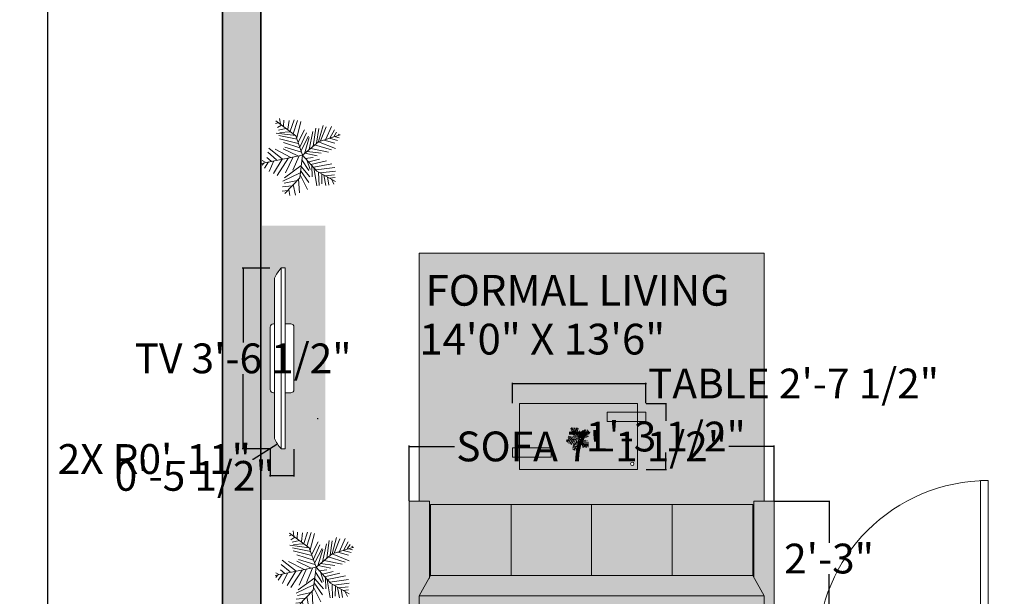
# Model space of a CAD drawing. Units: inches. Extents: x 2167 to 2589, y 1680 to 2489.
# Tile 31 of 38: x 2167 to 2399, y 1865 to 2000. Entities that reach past the tile are written whole.
import ezdxf

# ---------------------------------------------------------------- set-up
doc = ezdxf.new("R2010")
doc.units = ezdxf.units.IN
doc.header["$MEASUREMENT"] = 0
doc.layers.get('0').update_dxf_attribs({"color": 250})
for name, color, linetype, lineweight in [('A-ANNO-DIMS', 2, 'Continuous', 18), ('A-AREA-IDEN', 7, 'Continuous', 18), ('A-DOOR', 4, 'Continuous', 18), ('A-EQPM', 34, 'Continuous', 18), ('A-FURN-PATT', 31, 'Continuous', 13), ('A-WALL-PATT', 250, 'Continuous', 13), ('C-PROP', 7, 'Continuous', 35), ('furniture', 34, 'Continuous', 18), ('L-PLNT', 106, 'Continuous', 13), ('walls', 7, 'Continuous', 35)]:
    doc.layers.add(name, color=color, linetype=linetype, lineweight=lineweight)
doc.layers.add('A-FURN-FIXD-PATT', color=33, linetype='Continuous', lineweight=13, true_color=0xcd8e5c)
doc.styles.get("Standard").update_dxf_attribs({"font": 'arial.ttf'})
doc.dimstyles.get("Standard").update_dxf_attribs({"dimtxt": 7, "dimasz": 0.18, "dimexe": 0.18, "dimexo": 0.0625, "dimgap": 0.09, "dimtad": 0, "dimtih": 1, "dimtoh": 1, "dimdec": 1, "dimzin": 0, "dimdsep": 46, "dimlunit": 3, "dimtxsty": 'Standard', "dimcen": 0.09, "dimadec": 0, "dimazin": 0, "dimtfac": 1, "dimtdec": 1, "dimtofl": 0, "dimtmove": 0, "dimatfit": 3, "dimfxl": 1, "dimtolj": 1, "dimtzin": 0, "dimarcsym": 0})

# ---------------------------------------------------------------- blocks, each defined once
blk = doc.blocks.new('*U2')
for p, q in [((0, 0), (0, -6)), ((40, 0), (40, -6))]:
    blk.add_line(p, q)
blk.add_lwpolyline([(0, 0), (0, 40), (1.75, 40), (1.75, 0)], close=True)
blk.add_arc((0, 0), 40, 0, 90)
blk = doc.blocks.new('PLASMA-LARGE')
at = {"layer": 'furniture'}
for p, q in [((-7.26, 0), (7.26, 0)), ((-18.61, -1), (18.61, -1)), ((-8, -1), (-8, -0.74)), ((8, -1), (8, -0.74)), ((-21, -2.5), (21, -2.5)), ((-21, -2.5), (-21, -3.5)), ((-21, -3.5), (21, -3.5)), ((-8, -3.5), (-8, -4.76)), ((8, -3.5), (8, -4.76)), ((21, -2.5), (21, -3.5)), ((-7.26, -5.5), (7.26, -5.5))]:
    blk.add_line(p, q, dxfattribs=at)
for centre, radius, start, end in [((-7.26, -0.74), 0.744, 90, 180), ((7.26, -0.74), 0.744, 0, 90), ((-13.97, -11.05), 11.07, 114.7602, 129.4175), ((13.97, -11.05), 11.07, 50.5825, 65.2398), ((-7.26, -4.76), 0.744, 180, 270), ((7.26, -4.76), 0.744, 270, 0)]:
    blk.add_arc(centre, radius, start, end, dxfattribs=at)
blk = doc.blocks.new('FABRIC SOFA 4S')
at = {"layer": 'furniture'}
for p, q in [((3, 54), (34, 54)), ((3, 51), (3, 54)), ((34, 48), (34, 54)), ((0, -51), (0, 51)), ((6, 51), (0, 51)), ((6, -51), (6, 51)), ((12, 47.63), (6, 51)), ((11.14, 48), (34, 48)), ((33, 23.81), (12, 23.81)), ((33, 0), (12, 0)), ((33, -23.81), (12, -23.81)), ((6, -51), (12, -47.63)), ((11.54, -48), (34, -48)), ((34, -48), (34, -54)), ((6, -51), (0, -51)), ((3, -54), (3, -51)), ((3, -54), (34, -54))]:
    blk.add_line(p, q, dxfattribs=at)
blk.add_lwpolyline([(12, -47.63), (12, 47.63), (33, 47.63), (33, -47.63)], close=True, dxfattribs=at)
blk = doc.blocks.new('tpoy')
at = {"layer": 'furniture'}
h = blk.add_hatch(color=256, dxfattribs=at)
h.dxf.hatch_style = 1
h.paths.add_polyline_path([(278.09, -251.06), (275.9, -251.06), (275.9, -258.19), (278.09, -258.19)])
h.paths.add_polyline_path([(278.09, -249.1), (275.9, -249.1), (275.9, -251.06), (278.09, -251.06)])
h.paths.add_polyline_path([(286.44, -271.28), (284.25, -271.28), (284.25, -278.76), (286.44, -278.76)])
h.paths.add_polyline_path([(286.44, -278.76), (284.25, -278.76), (284.25, -280.38), (286.44, -280.38)])
for p, q in [((275.9, -249.1), (278.09, -249.1)), ((275.9, -258.19), (275.9, -249.1)), ((278.09, -249.1), (278.09, -258.19)), ((273.86, -251.06), (273.86, -278.76)), ((289.38, -251.06), (273.86, -251.06)), ((289.38, -278.76), (289.38, -251.06)), ((278.09, -258.19), (275.9, -258.19)), ((284.25, -280.38), (284.25, -271.28)), ((286.44, -271.28), (286.44, -280.38)), ((273.86, -278.76), (289.38, -278.76))]:
    blk.add_line(p, q, dxfattribs=at)
blk.add_circle((288.03, -252.28), 0.401, dxfattribs=at)
blk = doc.blocks.new('*U8')
for p, q in [((-10.186, 53.64), (-13.084, 55.962)), ((0, 0), (-10.5, 57)), ((-9.099, 51.782), (-6.563, 55.962)), ((-7.288, 39.707), (-21.778, 46.673)), ((-8.737, 47.138), (-17.069, 52.711)), ((-7.65, 43.423), (-2.578, 49.46)), ((-5.839, 35.992), (4.667, 48.067)), ((-5.114, 27.632), (10.463, 46.673)), ((-48.585, 21.131), (-49.309, 29.026)), ((-43.513, 28.561), (-42.427, 15.558)), ((-35.544, 28.097), (-24.314, 3.947)), ((-3.665, 19.273), (-27.574, 35.527)), ((-5.114, 28.097), (-24.676, 40.636)), ((-2.941, 16.486), (8.652, 37.85)), ((16.259, 5.805), (23.142, 31.348)), ((22.055, 7.198), (27.489, 32.277)), ((27, 9), (48, 36)), ((27.127, 9.056), (31.112, 35.992)), ((31.836, 30.883), (32.561, 16.486)), ((35.096, 32.741), (37.27, 22.524)), ((38.719, 34.134), (41.979, 28.561)), ((43.791, 29.954), (51.036, 30.883)), ((44.153, 36.456), (45.239, 32.741)), ((-47.498, 19.737), (-55.83, 18.344)), ((-40.615, 13.7), (-55.105, 10.913)), ((-31.5, 4.5), (-52.5, 25.5)), ((-38.442, 26.239), (-34.819, 7.663)), ((-14.533, 2.09), (-30.834, 25.31)), ((-24.314, 23.917), (-2.941, 13.7)), ((-20.691, 13.7), (-1.129, 4.876)), ((-1.129, 6.734), (9.014, 26.704)), ((3.942, 1.625), (11.187, 24.381)), ((10.101, 3.483), (17.708, 26.239)), ((33.285, 16.486), (48.862, 10.913)), ((36.183, 19.737), (48.137, 17.88)), ((40.53, 25.775), (48.862, 24.846)), ((-33.37, 6.269), (-52.207, 5.34)), ((-28.299, 3.483), (-47.86, -5.805)), ((-21.416, 3.018), (-38.079, -8.128)), ((0, 0), (-31.5, 4.5)), ((-15.982, 2.09), (-30.11, -9.521)), ((0, 0), (-22.5, -19.5)), ((-6.563, 1.161), (-21.416, -8.128)), ((0, 0), (27, 9)), ((0, 0), (18, -22.5)), ((6.478, 1.625), (26.04, -8.592)), ((11.187, 3.483), (30.749, -5.805)), ((18.07, 5.805), (35.096, -3.483)), ((24.229, 7.663), (46.688, 1.625)), ((29.662, 12.307), (48.137, 6.269)), ((-15.257, -12.772), (-30.11, -12.772)), ((-6.563, -5.805), (-19.967, -9.985)), ((-13.446, -11.378), (-8.737, -32.741)), ((-9.461, -8.592), (-6.201, -23.453)), ((-4.752, -3.483), (-3.665, -14.629)), ((2.493, -3.019), (-1.491, -20.202)), ((1.769, -2.555), (24.229, -9.521)), ((5.029, -6.27), (2.131, -25.775)), ((9.014, -11.378), (3.58, -35.992)), ((7.565, -9.056), (32.198, -14.629)), ((-17.431, -15.094), (-42.789, -18.809)), ((-24.314, -21.596), (-42.427, -22.06)), ((-26.849, -26.24), (-40.253, -25.775)), ((-22.5, -19.5), (-37.5, -45)), ((-25.038, -23.918), (-22.865, -45.281)), ((-20.691, -18.345), (-17.793, -44.352)), ((-17.069, -15.094), (-12.721, -40.172)), ((14.085, -16.951), (6.478, -40.172)), ((18.07, -22.524), (8.289, -45.745)), ((12.274, -15.094), (36.907, -18.809)), ((16.259, -19.738), (36.183, -22.989)), ((18, -22.5), (27, -52.5)), ((18.433, -22.524), (40.53, -29.026)), ((19.157, -25.311), (38.719, -33.206)), ((-28.299, -29.026), (-42.789, -31.348)), ((-30.834, -34.135), (-42.427, -35.528)), ((-34.457, -39.708), (-40.978, -42.494)), ((-32.646, -36.921), (-31.921, -44.352)), ((-29.023, -30.884), (-27.936, -43.887)), ((20.244, -30.419), (15.897, -44.816)), ((22.78, -37.85), (19.519, -48.532)), ((21.331, -32.741), (39.081, -40.636)), ((22.78, -38.314), (34.372, -44.816)), ((24.591, -45.745), (23.142, -50.854)), ((24.591, -43.423), (30.749, -47.603)), ((26.764, -49.925), (28.213, -50.854))]:
    blk.add_line(p, q)
blk = doc.blocks.new('*D24')
at = {"layer": 'A-ANNO-DIMS', "color": 0, "lineweight": -2, "transparency": 16777216}
for p, q in [((2174.43, 2407.69), (2173.89, 2407.69)), ((2174.07, 2407.51), (2174.07, 2051.36)), ((2174.07, 1687.87), (2174.07, 2044.03)), ((2174.43, 1687.69), (2173.89, 1687.69))]:
    blk.add_line(p, q, dxfattribs=at)
at = {"layer": 'A-ANNO-DIMS', "color": 0, "transparency": 16777216}
for points in [[(2174.04, 2407.51), (2174.1, 2407.51), (2174.07, 2407.69)], [(2174.04, 1687.87), (2174.1, 1687.87), (2174.07, 1687.69)]]:
    blk.add_solid(points, dxfattribs=at)
at = {"layer": 'Defpoints', "color": 0, "transparency": 16777216}
for p in [(2174.49, 2407.69), (2174.07, 1687.69), (2174.49, 1687.69)]:
    blk.add_point(p, dxfattribs=at)
at = {"layer": 'A-ANNO-DIMS', "color": 0, "transparency": 16777216, "insert": (2174.07, 2047.69), "char_height": 7, "attachment_point": 5}
blk.add_mtext("\\A1;60'", dxfattribs=at)
blk = doc.blocks.new('*D39')
at = {"layer": 'A-ANNO-DIMS', "color": 0, "lineweight": -2, "transparency": 16777216}
for p, q in [((2258.86, 1887.26), (2258.86, 1900.24)), ((2259.04, 1900.06), (2269.52, 1900.06)), ((2344.41, 1900.06), (2333.93, 1900.06)), ((2344.59, 1887.26), (2344.59, 1900.24))]:
    blk.add_line(p, q, dxfattribs=at)
at = {"layer": 'A-ANNO-DIMS', "color": 0, "transparency": 16777216}
for points in [[(2259.04, 1900.09), (2259.04, 1900.03), (2258.86, 1900.06)], [(2344.41, 1900.09), (2344.41, 1900.03), (2344.59, 1900.06)]]:
    blk.add_solid(points, dxfattribs=at)
at = {"layer": 'Defpoints', "color": 0, "transparency": 16777216}
for p in [(2258.86, 1900.06), (2258.86, 1887.2), (2344.59, 1887.2)]:
    blk.add_point(p, dxfattribs=at)
at = {"layer": 'A-ANNO-DIMS', "color": 0, "transparency": 16777216, "insert": (2301.72, 1900.06), "char_height": 7, "attachment_point": 5}
blk.add_mtext('\\A1;SOFA 7\'-1 1/2"', dxfattribs=at)
blk = doc.blocks.new('*D40')
at = {"layer": 'A-ANNO-DIMS', "color": 0, "lineweight": -2, "transparency": 16777216}
for p, q in [((2344.65, 1887.2), (2357.62, 1887.2)), ((2357.44, 1887.02), (2357.44, 1877.38)), ((2357.44, 1860.4), (2357.44, 1870.04)), ((2344.65, 1860.22), (2357.62, 1860.22))]:
    blk.add_line(p, q, dxfattribs=at)
at = {"layer": 'A-ANNO-DIMS', "color": 0, "transparency": 16777216}
for points in [[(2357.41, 1887.02), (2357.47, 1887.02), (2357.44, 1887.2)], [(2357.41, 1860.4), (2357.47, 1860.4), (2357.44, 1860.22)]]:
    blk.add_solid(points, dxfattribs=at)
at = {"layer": 'Defpoints', "color": 0, "transparency": 16777216}
for p in [(2344.59, 1887.2), (2357.44, 1887.2), (2344.59, 1860.22)]:
    blk.add_point(p, dxfattribs=at)
at = {"layer": 'A-ANNO-DIMS', "color": 0, "transparency": 16777216, "insert": (2357.44, 1873.71), "char_height": 7, "attachment_point": 5}
blk.add_mtext('\\A1;2\'-3"', dxfattribs=at)
blk = doc.blocks.new('*D55')
at = {"layer": 'A-ANNO-DIMS', "color": 0, "lineweight": -2, "transparency": 16777216}
for p, q in [((2226.2, 1941.98), (2219.71, 1941.98)), ((2219.89, 1941.8), (2219.89, 1924.46)), ((2219.89, 1899.69), (2219.89, 1917.03)), ((2226.2, 1899.51), (2219.71, 1899.51))]:
    blk.add_line(p, q, dxfattribs=at)
at = {"layer": 'A-ANNO-DIMS', "color": 0, "transparency": 16777216}
for points in [[(2219.86, 1941.8), (2219.92, 1941.8), (2219.89, 1941.98)], [(2219.86, 1899.69), (2219.92, 1899.69), (2219.89, 1899.51)]]:
    blk.add_solid(points, dxfattribs=at)
at = {"layer": 'Defpoints', "color": 0, "transparency": 16777216}
for p in [(2219.89, 1941.98), (2226.26, 1941.98), (2226.26, 1899.51)]:
    blk.add_point(p, dxfattribs=at)
at = {"layer": 'A-ANNO-DIMS', "color": 0, "transparency": 16777216, "insert": (2219.89, 1920.75), "char_height": 7, "attachment_point": 5}
blk.add_mtext('\\A1;TV 3\'-6 1/2"', dxfattribs=at)
blk = doc.blocks.new('*D56')
at = {"layer": 'A-ANNO-DIMS', "color": 0, "lineweight": -2, "transparency": 16777216}
for p, q in [((2226.26, 1899.45), (2226.26, 1892.96)), ((2231.82, 1899.45), (2231.82, 1892.96)), ((2226.26, 1893.14), (2226.08, 1893.14)), ((2231.64, 1893.14), (2226.44, 1893.14))]:
    blk.add_line(p, q, dxfattribs=at)
at = {"layer": 'A-ANNO-DIMS', "color": 0, "transparency": 16777216}
for points in [[(2226.44, 1893.17), (2226.44, 1893.11), (2226.26, 1893.14)], [(2231.64, 1893.17), (2231.64, 1893.11), (2231.82, 1893.14)]]:
    blk.add_solid(points, dxfattribs=at)
at = {"layer": 'Defpoints', "color": 0, "transparency": 16777216}
for p in [(2226.26, 1899.51), (2231.82, 1899.51), (2226.26, 1893.14)]:
    blk.add_point(p, dxfattribs=at)
at = {"layer": 'A-ANNO-DIMS', "color": 0, "transparency": 16777216, "insert": (2208.53, 1893.14), "char_height": 7, "attachment_point": 5}
blk.add_mtext('\\A1;0\'-5 1/2"', dxfattribs=at)
blk = doc.blocks.new('*D57')
at = {"layer": 'A-ANNO-DIMS', "color": 0, "lineweight": -2, "transparency": 16777216}
for p, q in [((2283.15, 1910.21), (2283.15, 1915.02)), ((2283.33, 1914.84), (2314.25, 1914.84)), ((2314.43, 1910.21), (2314.43, 1915.02)), ((2314.43, 1914.84), (2314.61, 1914.84))]:
    blk.add_line(p, q, dxfattribs=at)
at = {"layer": 'A-ANNO-DIMS', "color": 0, "transparency": 16777216}
for points in [[(2283.33, 1914.87), (2283.33, 1914.81), (2283.15, 1914.84)], [(2314.25, 1914.87), (2314.25, 1914.81), (2314.43, 1914.84)]]:
    blk.add_solid(points, dxfattribs=at)
at = {"layer": 'Defpoints', "color": 0, "transparency": 16777216}
for p in [(2314.43, 1914.84), (2283.15, 1910.15), (2314.43, 1910.15)]:
    blk.add_point(p, dxfattribs=at)
at = {"layer": 'A-ANNO-DIMS', "color": 0, "transparency": 16777216, "insert": (2349.1, 1914.84), "char_height": 7, "attachment_point": 5}
blk.add_mtext('\\A1;TABLE 2\'-7 1/2"', dxfattribs=at)
blk = doc.blocks.new('*D58')
at = {"layer": 'A-ANNO-DIMS', "color": 0, "lineweight": -2, "transparency": 16777216}
for p, q in [((2314.49, 1910.15), (2319.3, 1910.15)), ((2319.12, 1909.97), (2319.12, 1906.1)), ((2319.12, 1894.8), (2319.12, 1898.67)), ((2314.49, 1894.62), (2319.3, 1894.62))]:
    blk.add_line(p, q, dxfattribs=at)
at = {"layer": 'A-ANNO-DIMS', "color": 0, "transparency": 16777216}
for points in [[(2319.09, 1909.97), (2319.15, 1909.97), (2319.12, 1910.15)], [(2319.09, 1894.8), (2319.15, 1894.8), (2319.12, 1894.62)]]:
    blk.add_solid(points, dxfattribs=at)
at = {"layer": 'Defpoints', "color": 0, "transparency": 16777216}
for p in [(2314.43, 1910.15), (2314.43, 1894.62), (2319.12, 1894.62)]:
    blk.add_point(p, dxfattribs=at)
at = {"layer": 'A-ANNO-DIMS', "color": 0, "transparency": 16777216, "insert": (2319.12, 1902.38), "char_height": 7, "attachment_point": 5}
blk.add_mtext('\\A1;1\'-3 1/2"', dxfattribs=at)
blk = doc.blocks.new('*D60')
at = {"layer": 'A-ANNO-DIMS', "color": 0, "lineweight": -2, "transparency": 16777216}
for p, q in [((2237.35, 1906.62), (2237.53, 1906.62)), ((2237.44, 1906.53), (2237.44, 1906.71)), ((2222.27, 1897.1), (2227.8, 1900.57)), ((2222.09, 1897.1), (2222.27, 1897.1))]:
    blk.add_line(p, q, dxfattribs=at)
at = {"layer": 'A-ANNO-DIMS', "color": 0, "transparency": 16777216}
blk.add_solid([(2227.79, 1900.6), (2227.82, 1900.55), (2227.95, 1900.67)], dxfattribs=at)
at = {"layer": 'Defpoints', "color": 0, "transparency": 16777216}
for p in [(2237.44, 1906.62), (2227.95, 1900.67)]:
    blk.add_point(p, dxfattribs=at)
at = {"layer": 'A-ANNO-DIMS', "color": 0, "transparency": 16777216, "insert": (2199.04, 1897.1), "char_height": 7, "attachment_point": 5}
blk.add_mtext('\\A1;2X R0\'-11"', dxfattribs=at)

msp = doc.modelspace()

# ---------------------------------------------------------------- hatches: boundary and pattern name
at = {"layer": 'A-FURN-FIXD-PATT'}
h = msp.add_hatch(color=256, dxfattribs=at)
h.dxf.hatch_style = 1
h.paths.add_polyline_path([(2239.21, 1951.93), (2224.31, 1951.93), (2224.31, 1887.49), (2239.21, 1887.49)])
h.paths.add_polyline_path([(2229.8, 1899.51), (2228.79, 1899.51, -0.064042), (2227.27, 1901.93), (2227.27, 1912.66), (2227.02, 1912.66, -0.414214), (2226.26, 1913.41), (2226.26, 1928.08, -0.414214), (2227.02, 1928.84), (2227.27, 1928.84), (2227.27, 1939.56, -0.064042), (2228.79, 1941.98), (2229.8, 1941.98), (2229.8, 1928.84), (2231.07, 1928.84, -0.414214), (2231.82, 1928.08), (2231.82, 1913.41, -0.414214), (2231.07, 1912.66), (2229.8, 1912.66)], flags=16)
at = {"layer": 'A-FURN-PATT'}
h = msp.add_hatch(color=256, dxfattribs=at)
h.dxf.hatch_style = 1
h.paths.add_polyline_path([(2342.2, 1945.44), (2261.25, 1945.44), (2261.25, 1887.2), (2263.63, 1887.2), (2263.63, 1869.21), (2261.25, 1864.98), (2342.2, 1864.98), (2339.82, 1869.21), (2339.82, 1887.2), (2342.2, 1887.2)])
h.paths.add_polyline_path([(2312.47, 1910.15), (2312.47, 1908.11), (2314.43, 1908.11), (2314.43, 1905.92), (2312.47, 1905.92), (2312.47, 1894.62), (2284.77, 1894.62), (2284.77, 1897.56), (2283.15, 1897.56), (2283.15, 1899.76), (2284.77, 1899.76), (2284.77, 1910.15)], flags=16)
h.paths.add_polyline_path([(2311.65, 1895.98, -1), (2310.85, 1895.98, -1)], flags=0)
h.paths.add_polyline_path([(2339.53, 1886.41), (2339.53, 1869.74), (2263.92, 1869.74), (2263.92, 1886.41)], flags=16)
h = msp.add_hatch(color=256, dxfattribs=at)
h.dxf.hatch_style = 1
h.paths.add_polyline_path([(2312.47, 1905.92), (2305.34, 1905.92), (2305.34, 1908.11), (2312.47, 1908.11), (2312.47, 1910.15), (2284.77, 1910.15), (2284.77, 1899.76), (2292.24, 1899.76), (2292.24, 1897.56), (2284.77, 1897.56), (2284.77, 1894.62), (2312.47, 1894.62)])
h.paths.add_polyline_path([(2300.61, 1903.15), (2300.62, 1903.15), (2300.62, 1903.16)], flags=16)
h.paths.add_polyline_path([(2298.68, 1901.96), (2297.25, 1901.67), (2297.26, 1901.69), (2297.28, 1901.68), (2298.68, 1901.96), (2298.2, 1903.33), (2298.19, 1903.34), (2298.2, 1903.34), (2298.68, 1901.96), (2298.82, 1902.07), (2298.82, 1902.09), (2298.84, 1902.09), (2298.68, 1901.96), (2299.46, 1901.1), (2299.47, 1901.1), (2299.47, 1901.08)], flags=16)
h.paths.add_polyline_path([(2311.65, 1895.98, -1), (2310.85, 1895.98, -1)], flags=16)
h = msp.add_hatch(color=256, dxfattribs=at)
h.dxf.hatch_style = 1
h.paths.add_polyline_path([(2263.92, 1886.41), (2263.92, 1869.74), (2282.82, 1869.74), (2282.82, 1886.41)])
h.paths.add_polyline_path([(2282.82, 1886.41), (2282.82, 1869.74), (2301.72, 1869.74), (2301.72, 1886.41)])
h.paths.add_polyline_path([(2301.72, 1886.41), (2301.72, 1869.74), (2320.63, 1869.74), (2320.63, 1886.41)])
h.paths.add_polyline_path([(2320.63, 1886.41), (2320.63, 1869.74), (2339.53, 1869.74), (2339.53, 1886.41)])
h.paths.add_polyline_path([(2263.92, 1869.74), (2261.25, 1864.98), (2342.2, 1864.98), (2339.53, 1869.74)])
h.paths.add_polyline_path([(2261.25, 1864.98), (2261.25, 1860.22), (2342.2, 1860.22), (2342.2, 1864.98)])
h.paths.add_polyline_path([(2258.86, 1887.2), (2258.86, 1862.6), (2261.25, 1862.6), (2261.25, 1864.98), (2263.63, 1869.21), (2263.63, 1887.2)])
h.paths.add_polyline_path([(2339.82, 1887.2), (2339.82, 1869.21), (2342.2, 1864.98), (2342.2, 1862.6), (2344.59, 1862.6), (2344.59, 1887.2)])
at = {"layer": 'A-WALL-PATT'}
h = msp.add_hatch(color=256, dxfattribs=at)
h.dxf.hatch_style = 1
h.paths.add_polyline_path([(2274.74, 1855.04), (2224.05, 1855.04), (2224.05, 2003.12), (2215.05, 2003.12), (2215.05, 1846.04), (2274.74, 1846.04)])
h.paths.add_polyline_path([(2354.89, 1855.04), (2330.89, 1855.04), (2330.89, 1846.04), (2354.77, 1846.04), (2354.77, 1852.04, -0.01877)])
h.paths.add_polyline_path([(2422.05, 1864.69), (2426.21, 1864.69), (2426.21, 1867.92), (2426.21, 1869.19), (2422.05, 1869.19), (2422.05, 1916.24), (2417.55, 1916.24), (2417.55, 1855.04), (2394.77, 1855.04), (2394.77, 1852.04), (2394.77, 1846.04), (2417.55, 1846.04), (2417.55, 1779.19), (2427.74, 1779.19), (2427.74, 1783.94), (2427.74, 1788.19), (2422.05, 1788.19)])

# ---------------------------------------------------------------- linework, layer by layer
at = {"layer": 'C-PROP'}
msp.add_line((2215.05, 1687.69), (2215.05, 2407.69), dxfattribs=at)
at = {"layer": 'furniture'}
for p, q in [((2261.25, 1887.2), (2261.25, 1945.44)), ((2261.25, 1945.44), (2342.2, 1945.44)), ((2342.2, 1945.44), (2342.2, 1887.2)), ((2283.15, 1897.56), (2283.15, 1899.76)), ((2292.24, 1899.76), (2292.24, 1897.56))]:
    msp.add_line(p, q, dxfattribs=at)
at = {"layer": 'walls'}
msp.add_line((2224.05, 1855.04), (2224.05, 2151.19), dxfattribs=at)

# ---------------------------------------------------------------- block references
at = {"layer": 'A-DOOR', "xscale": -1}
msp.add_blockref('*U2', (2394.77, 1852.04), dxfattribs=at)
at = {"layer": 'A-EQPM', "xscale": 1.011294184530666, "yscale": 1.011294184530666, "zscale": 1.011294184530666, "rotation": 90.00000000000003}
msp.add_blockref('PLASMA-LARGE', (2226.26, 1920.75), dxfattribs=at)
at = {"layer": 'furniture', "rotation": 270}
msp.add_blockref('tpoy', (2563.53, 2184), dxfattribs=at)
at = {"layer": 'furniture', "xscale": 0.7937147270336093, "yscale": 0.7937147270336093, "zscale": 0.7937147270336093, "rotation": 90}
msp.add_blockref('FABRIC SOFA 4S', (2301.72, 1860.22), dxfattribs=at)
at = {"layer": 'L-PLNT', "rotation": 90.98387132377816}
for p, xscale, yscale, zscale in [((2233.85, 1968.52), 0.1698531738429223, 0.1698531738429223, 0.1698531738429223), ((2298.68, 1901.96), 0.0510892351028333, 0.0510892351028333, 0.0510892351028333), ((2237.04, 1871.66), 0.1698531738429223, 0.1698531738429223, 0.1698531738429223)]:
    msp.add_blockref('*U8', p, dxfattribs=dict(at, xscale=xscale, yscale=yscale, zscale=zscale))

# ---------------------------------------------------------------- texts
at = {"layer": 'A-AREA-IDEN'}
for s, p in [('FORMAL LIVING', (2262.72, 1933.13)), ('14\'0" X 13\'6"', (2261.25, 1921.66))]:
    msp.add_text(s, height=7.2272, dxfattribs=at).set_placement(p)

# ---------------------------------------------------------------- dimensions: what is measured, and where the dimension line sits
at = {"layer": 'A-ANNO-DIMS'}
for base, p1, p2, angle, override, picture, middle in [((2174.07, 1687.69), (2174.49, 2407.69), (2174.49, 1687.69), 90, {"dimclrd": 0, "dimclre": 0, "dimclrt": 0}, '*D24', (2174.07, 2047.69)), ((2319.12, 1894.62), (2314.43, 1910.15), (2314.43, 1894.62), 270, {"dimdec": 1, "dimlfac": 1, "dimrnd": 0, "dimzin": 1, "dimdsep": 46, "dimlunit": 4, "dimfrac": 2}, '*D58', (2319.12, 1902.38)), ((2226.26, 1893.14), (2231.82, 1899.51), (2226.26, 1899.51), 180, {"dimdec": 1, "dimlfac": 1, "dimrnd": 0, "dimzin": 1, "dimdsep": 46, "dimlunit": 4, "dimfrac": 2}, '*D56', (2208.53, 1893.14)), ((2357.44, 1887.2), (2344.59, 1860.22), (2344.59, 1887.2), 90, {"dimdec": 1, "dimlfac": 1, "dimrnd": 0, "dimzin": 1, "dimdsep": 46, "dimlunit": 4, "dimfrac": 2}, '*D40', (2357.44, 1873.71))]:
    dim = msp.add_linear_dim(base=base, p1=p1, p2=p2, angle=angle, dimstyle='Standard', override=override, dxfattribs=at)
    dim.commit()
    dim.dimension.update_dxf_attribs({"geometry": picture, "text_midpoint": middle})
for base, p1, p2, angle, text, picture, middle in [((2219.89, 1941.98), (2226.26, 1899.51), (2226.26, 1941.98), 90, 'TV <>', '*D55', (2219.89, 1920.75)), ((2258.86, 1900.06), (2344.59, 1887.2), (2258.86, 1887.2), 180, 'SOFA <>', '*D39', (2301.72, 1900.06))]:
    dim = msp.add_linear_dim(base=base, p1=p1, p2=p2, angle=angle, text=text, dimstyle='Standard', override={"dimdec": 1, "dimlfac": 1, "dimrnd": 0, "dimzin": 1, "dimdsep": 46, "dimlunit": 4, "dimfrac": 2}, dxfattribs=at)
    dim.commit()
    dim.dimension.update_dxf_attribs({"geometry": picture, "text_midpoint": middle})
dim = msp.add_linear_dim(base=(2314.43, 1914.84), p1=(2283.15, 1910.15), p2=(2314.43, 1910.15), text='TABLE <>', dimstyle='Standard', override={"dimdec": 1, "dimlfac": 1, "dimrnd": 0, "dimzin": 1, "dimdsep": 46, "dimlunit": 4, "dimfrac": 2}, dxfattribs=at)
dim.commit()
dim.dimension.update_dxf_attribs({"geometry": '*D57', "text_midpoint": (2349.1, 1914.84)})
dim = msp.add_radius_dim(center=(2237.44, 1906.62), mpoint=(2227.95, 1900.67), text='2X <>', dimstyle='Standard', override={"dimdec": 1, "dimlfac": 1, "dimrnd": 0, "dimzin": 1, "dimdsep": 46, "dimlunit": 4, "dimfrac": 2}, dxfattribs=at)
dim.commit()
dim.dimension.update_dxf_attribs({"geometry": '*D60', "text_midpoint": (2199.04, 1897.1), "dimtype": 164})

doc.saveas('drawing.dxf')
